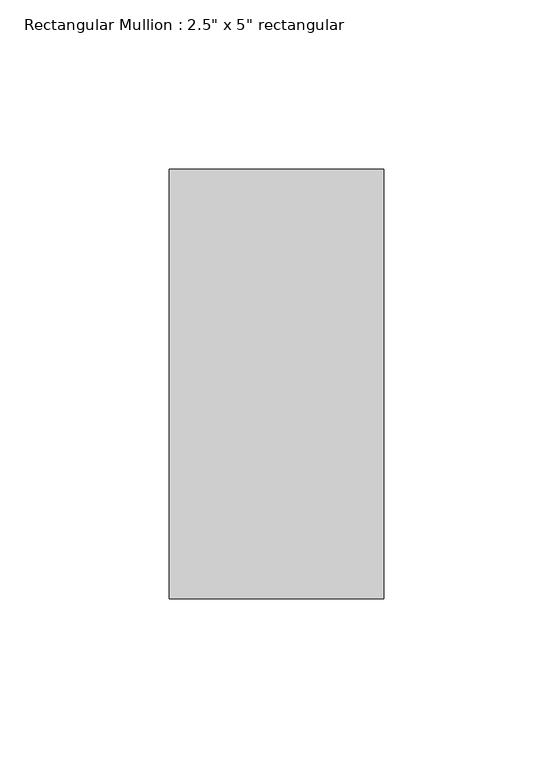
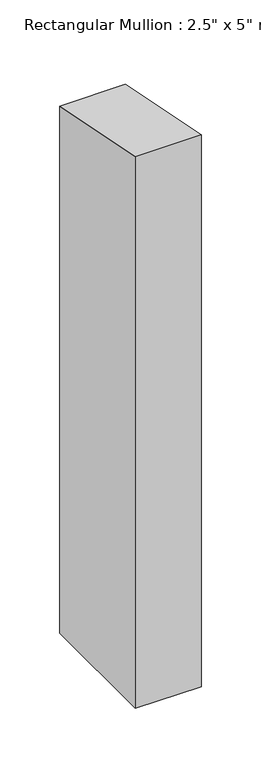
"""IFC4 building model written with IfcOpenShell, lengths in millimetres: member geometry."""

from ifc_helpers import new_model, si_unit, frame, origin, place, context, project, spatial, polyline, outline, extrude, source, transform, mapped, element, save


def member_4115b715(model_context):
    return source(origin(), model_context, "Body", "SweptSolid", [
        extrude(outline(polyline([(-63.5, 12.6309353), (63.5, -12.6309353), (63.5, -551.8845736), (-63.5, -551.8845736), (-63.5, 12.6309353)])), frame((-63.5, 0.0, 0.0), z_axis=(1.0, 0.0, 0.0), x_axis=(0.0, 1.0, 0.0)), (0.0, 0.0, 1.0), 63.5),
    ])


if __name__ == "__main__":
    model = new_model("IFC4")
    model_context = context("Model", 3, world=origin())
    ifc_project = project(units=[si_unit("LENGTHUNIT", "METRE", prefix="MILLI")], contexts=[model_context])
    site = spatial("IfcSite", under=ifc_project)
    building = spatial("IfcBuilding", under=site)
    placement = place(None, origin())
    member_shape = member_4115b715(model_context)
    element("IfcMember", 1, ObjectType="Rectangular Mullion : 2.5\" x 5\" rectangular", at=placement, inside=building, context=model_context, shape_type="MappedRepresentation", body=[
        mapped(member_shape, transform((0.0, 0.0, 0.0), x_axis=(1.0, 0.0, 0.0), y_axis=(0.0, 1.0, 0.0), z_axis=(0.0, 0.0, 1.0))),
    ])
    save(model, "model.ifc")

# Revit data of these elements
# Type "Rectangular Mullion : 2.5\" x 5\" rectangular"
#   built-in parameter 1007304 = 0.416667 (stored number, unit not read)
#   built-in parameter 1007301 = 0.104167 (stored number, unit not read)
#   built-in parameter 1007300 = 0.104167 (stored number, unit not read)
# Element 1 (IfcMember, "Rectangular Mullion : 2.5\" x 5\" rectangular")
#   Materials on its faces: "Iron, Ductile"
# Materials
#   "Iron, Ductile": class "Metal", colour RGB 0 0 0, transparency 0, Description = "Ductile cast iron", Cost = 0
